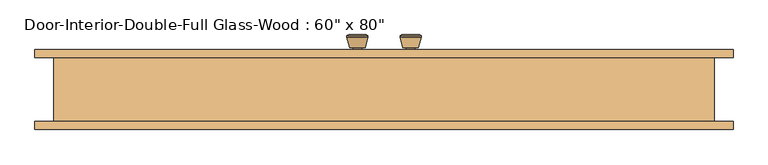
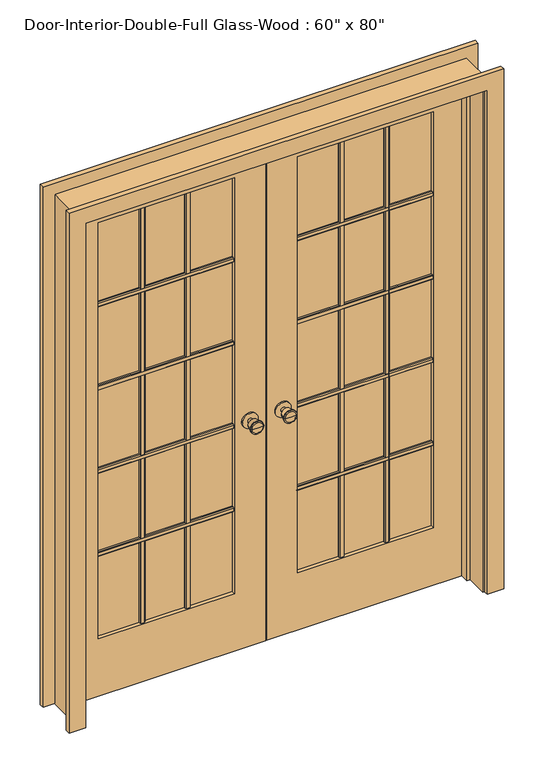
"""IFC4 building model written with IfcOpenShell, lengths in millimetres: door geometry."""

from ifc_helpers import new_model, si_unit, point, frame, frame_2d, origin, place, context, project, spatial, polyline, circle_curve, trimmed, segment, composite_curve, outline, extrude, faceted_brep, source, transform, mapped, element, save
from ifc_brep_helpers import plane_surface, cylinder_surface, revolved_surface, advanced_brep


def door_31a77bde(model_context):
    return source(origin(), model_context, "Body", "SolidModel", [
        advanced_brep(
        [(-63.5, 79.025, 914.4), (-73.5, 79.025, 914.4), (-53.5, 79.025, 914.4), (-83.9758676, 128.025, 914.4), (-63.5, 128.025, 914.4), (-43.0241324, 128.025, 914.4), (-88.5, 126.1971319, 914.4), (-38.5, 126.1971319, 914.4), (-88.5, 122.7334537, 914.4), (-38.5, 122.7334537, 914.4), (-82.136236, 98.025, 914.4), (-44.863764, 98.025, 914.4), (-73.5, 98.025, 914.4), (-53.5, 98.025, 914.4)],
        [
            (0, 1),
            (1, 2, circle_curve(frame((-63.5, 79.025, 914.4), z_axis=(0.0, -1.0, 0.0), x_axis=(1.0, 0.0, 0.0)), 10.0)),
            (2, 0),
            (2, 1, circle_curve(frame((-63.5, 79.025, 914.4), z_axis=(0.0, -1.0, 0.0), x_axis=(1.0, 0.0, 0.0)), 10.0)),
            (3, 4),
            (4, 5),
            (5, 3, circle_curve(frame((-63.5, 128.025, 914.4), z_axis=(0.0, 1.0, 0.0), x_axis=(1.0, 0.0, 0.0)), 20.4758676)),
            (3, 5, circle_curve(frame((-63.5, 128.025, 914.4), z_axis=(0.0, 1.0, 0.0), x_axis=(1.0, 0.0, 0.0)), 20.4758676)),
            (6, 3),
            (5, 7),
            (7, 6, circle_curve(frame((-63.5, 126.1971319, 914.4), z_axis=(0.0, 1.0, 0.0), x_axis=(1.0, 0.0, 0.0)), 25.0)),
            (6, 7, circle_curve(frame((-63.5, 126.1971319, 914.4), z_axis=(0.0, 1.0, 0.0), x_axis=(1.0, 0.0, 0.0)), 25.0)),
            (8, 6),
            (7, 9),
            (9, 8, circle_curve(frame((-63.5, 122.7334537, 914.4), z_axis=(0.0, 1.0, 0.0), x_axis=(1.0, 0.0, 0.0)), 25.0)),
            (8, 9, circle_curve(frame((-63.5, 122.7334537, 914.4), z_axis=(0.0, 1.0, 0.0), x_axis=(1.0, 0.0, 0.0)), 25.0)),
            (10, 8),
            (9, 11),
            (11, 10, circle_curve(frame((-63.5, 98.025, 914.4), z_axis=(0.0, 1.0, 0.0), x_axis=(1.0, 0.0, 0.0)), 18.636236)),
            (10, 11, circle_curve(frame((-63.5, 98.025, 914.4), z_axis=(0.0, 1.0, 0.0), x_axis=(1.0, 0.0, 0.0)), 18.636236)),
            (12, 10),
            (11, 13),
            (13, 12, circle_curve(frame((-63.5, 98.025, 914.4), z_axis=(0.0, 1.0, 0.0), x_axis=(1.0, 0.0, 0.0)), 10.0)),
            (12, 13, circle_curve(frame((-63.5, 98.025, 914.4), z_axis=(0.0, 1.0, 0.0), x_axis=(1.0, 0.0, 0.0)), 10.0)),
            (1, 12),
            (13, 2),
        ],
        [
            plane_surface(frame((-63.5, 79.025, 914.4), z_axis=(0.0, -1.0, 0.0), x_axis=(1.0, 0.0, 0.0))),
            plane_surface(frame((-63.5, 128.025, 914.4), z_axis=(0.0, 1.0, 0.0), x_axis=(1.0, 0.0, 0.0))),
            revolved_surface(polyline([(-43.0241324, 128.025, 914.4), (-38.5, 126.1971319, 914.4)]), (-63.5, 79.025, 914.4), (0.0, -1.0, 0.0)),
            cylinder_surface(frame((-63.5, 79.025, 914.4), z_axis=(0.0, -1.0, 0.0), x_axis=(1.0, 0.0, 0.0)), 25.0),
            revolved_surface(polyline([(-38.5, 122.7334537, 914.4), (-44.863764, 98.025, 914.4)]), (-63.5, 79.025, 914.4), (0.0, -1.0, 0.0)),
            plane_surface(frame((-63.5, 98.025, 914.4), z_axis=(0.0, -1.0, 0.0), x_axis=(1.0, 0.0, 0.0))),
            cylinder_surface(frame((-63.5, 79.025, 914.4), z_axis=(0.0, -1.0, 0.0), x_axis=(1.0, 0.0, 0.0)), 10.0),
        ],
        [
            (0, [[1, 2, 3]]),
            (0, [[-3, 4, -1]]),
            (1, [[5, 6, 7]]),
            (1, [[-6, -5, 8]]),
            (2, [[9, -7, 10, 11]]),
            (2, [[-10, -8, -9, 12]]),
            (3, [[13, -11, 14, 15]]),
            (3, [[-14, -12, -13, 16]]),
            (4, [[17, -15, 18, 19]]),
            (4, [[-18, -16, -17, 20]]),
            (5, [[21, -19, 22, 23]]),
            (5, [[-22, -20, -21, 24]]),
            (6, [[25, -23, 26, -2]]),
            (6, [[-26, -24, -25, -4]]),
        ],
    ),
        extrude(outline(composite_curve([segment(trimmed(circle_curve(frame_2d((914.4, -63.5)), 30.0), [point((914.4, -33.5))], [point((914.4, -93.5))], False, "CARTESIAN"), True, "CONTINUOUS"), segment(trimmed(circle_curve(frame_2d((914.4, -63.5)), 30.0), [point((914.4, -93.5))], [point((914.4, -33.5))], False, "CARTESIAN"), True, "CONTINUOUS")], self_intersect=False)), frame((0.0, 73.025, 0.0), z_axis=(0.0, 1.0, 0.0), x_axis=(0.0, 0.0, 1.0)), (0.0, 0.0, 1.0), 6.0),
        advanced_brep(
        [(-63.5, 32.1, 914.4), (-53.5, 32.1, 914.4), (-73.5, 32.1, 914.4), (-83.9758676, -16.9, 914.4), (-43.0241324, -16.9, 914.4), (-63.5, -16.9, 914.4), (-88.5, -15.0721319, 914.4), (-38.5, -15.0721319, 914.4), (-88.5, -11.6084537, 914.4), (-38.5, -11.6084537, 914.4), (-82.136236, 13.1, 914.4), (-44.863764, 13.1, 914.4), (-73.5, 13.1, 914.4), (-53.5, 13.1, 914.4)],
        [
            (0, 1),
            (1, 2, circle_curve(frame((-63.5, 32.1, 914.4), z_axis=(0.0, 1.0, 0.0), x_axis=(1.0, 0.0, 0.0)), 10.0)),
            (2, 0),
            (2, 1, circle_curve(frame((-63.5, 32.1, 914.4), z_axis=(0.0, 1.0, 0.0), x_axis=(1.0, 0.0, 0.0)), 10.0)),
            (3, 4, circle_curve(frame((-63.5, -16.9, 914.4), z_axis=(0.0, -1.0, 0.0), x_axis=(1.0, 0.0, 0.0)), 20.4758676)),
            (4, 5),
            (5, 3),
            (4, 3, circle_curve(frame((-63.5, -16.9, 914.4), z_axis=(0.0, -1.0, 0.0), x_axis=(1.0, 0.0, 0.0)), 20.4758676)),
            (6, 7, circle_curve(frame((-63.5, -15.0721319, 914.4), z_axis=(0.0, -1.0, 0.0), x_axis=(1.0, 0.0, 0.0)), 25.0)),
            (7, 4),
            (3, 6),
            (7, 6, circle_curve(frame((-63.5, -15.0721319, 914.4), z_axis=(0.0, -1.0, 0.0), x_axis=(1.0, 0.0, 0.0)), 25.0)),
            (8, 9, circle_curve(frame((-63.5, -11.6084537, 914.4), z_axis=(0.0, -1.0, 0.0), x_axis=(1.0, 0.0, 0.0)), 25.0)),
            (9, 7),
            (6, 8),
            (9, 8, circle_curve(frame((-63.5, -11.6084537, 914.4), z_axis=(0.0, -1.0, 0.0), x_axis=(1.0, 0.0, 0.0)), 25.0)),
            (10, 11, circle_curve(frame((-63.5, 13.1, 914.4), z_axis=(0.0, -1.0, 0.0), x_axis=(1.0, 0.0, 0.0)), 18.636236)),
            (11, 9),
            (8, 10),
            (11, 10, circle_curve(frame((-63.5, 13.1, 914.4), z_axis=(0.0, -1.0, 0.0), x_axis=(1.0, 0.0, 0.0)), 18.636236)),
            (12, 13, circle_curve(frame((-63.5, 13.1, 914.4), z_axis=(0.0, -1.0, 0.0), x_axis=(1.0, 0.0, 0.0)), 10.0)),
            (13, 11),
            (10, 12),
            (13, 12, circle_curve(frame((-63.5, 13.1, 914.4), z_axis=(0.0, -1.0, 0.0), x_axis=(1.0, 0.0, 0.0)), 10.0)),
            (1, 13),
            (12, 2),
        ],
        [
            plane_surface(frame((-63.5, 32.1, 914.4), z_axis=(0.0, 1.0, 0.0), x_axis=(1.0, 0.0, 0.0))),
            plane_surface(frame((-63.5, -16.9, 914.4), z_axis=(0.0, -1.0, 0.0), x_axis=(1.0, 0.0, 0.0))),
            revolved_surface(polyline([(-43.0241324, -16.9, 914.4), (-38.5, -15.0721319, 914.4)]), (-63.5, 32.1, 914.4), (0.0, 1.0, 0.0)),
            cylinder_surface(frame((-63.5, 32.1, 914.4), z_axis=(0.0, 1.0, 0.0), x_axis=(1.0, 0.0, 0.0)), 25.0),
            revolved_surface(polyline([(-38.5, -11.6084537, 914.4), (-44.863764, 13.1, 914.4)]), (-63.5, 32.1, 914.4), (0.0, 1.0, 0.0)),
            plane_surface(frame((-63.5, 13.1, 914.4), z_axis=(0.0, 1.0, 0.0), x_axis=(1.0, 0.0, 0.0))),
            cylinder_surface(frame((-63.5, 32.1, 914.4), z_axis=(0.0, 1.0, 0.0), x_axis=(1.0, 0.0, 0.0)), 10.0),
        ],
        [
            (0, [[1, 2, 3]]),
            (0, [[-3, 4, -1]]),
            (1, [[5, 6, 7]]),
            (1, [[8, -7, -6]]),
            (2, [[9, 10, -5, 11]]),
            (2, [[12, -11, -8, -10]]),
            (3, [[13, 14, -9, 15]]),
            (3, [[16, -15, -12, -14]]),
            (4, [[17, 18, -13, 19]]),
            (4, [[20, -19, -16, -18]]),
            (5, [[21, 22, -17, 23]]),
            (5, [[24, -23, -20, -22]]),
            (6, [[-2, 25, -21, 26]]),
            (6, [[-4, -26, -24, -25]]),
        ],
    ),
        extrude(outline(composite_curve([segment(trimmed(circle_curve(frame_2d((914.4, -63.5)), 30.0), [point((914.4, -33.5))], [point((914.4, -93.5))], False, "CARTESIAN"), True, "CONTINUOUS"), segment(trimmed(circle_curve(frame_2d((914.4, -63.5)), 30.0), [point((914.4, -93.5))], [point((914.4, -33.5))], False, "CARTESIAN"), True, "CONTINUOUS")], self_intersect=False)), frame((0.0, 32.1, 0.0), z_axis=(0.0, 1.0, 0.0), x_axis=(0.0, 0.0, 1.0)), (0.0, 0.0, 1.0), 6.0),
        extrude(outline(polyline([(52.07, 1586.23), (52.07, 1567.18), (45.72, 1567.18), (42.545, 1570.355), (42.545, 1583.055), (45.72, 1586.23), (52.07, 1586.23)])), frame((120.65, 0.0, 0.0), z_axis=(1.0, 0.0, 0.0), x_axis=(0.0, 1.0, 0.0)), (0.0, 0.0, 1.0), 520.7),
        extrude(outline(polyline([(52.07, 1249.9975), (52.07, 1230.9475), (45.72, 1230.9475), (42.545, 1234.1225), (42.545, 1246.8225), (45.72, 1249.9975), (52.07, 1249.9975)])), frame((120.65, 0.0, 0.0), z_axis=(1.0, 0.0, 0.0), x_axis=(0.0, 1.0, 0.0)), (0.0, 0.0, 1.0), 520.7),
        extrude(outline(polyline([(52.07, 913.765), (52.07, 894.715), (45.72, 894.715), (42.545, 897.89), (42.545, 910.59), (45.72, 913.765), (52.07, 913.765)])), frame((120.65, 0.0, 0.0), z_axis=(1.0, 0.0, 0.0), x_axis=(0.0, 1.0, 0.0)), (0.0, 0.0, 1.0), 520.7),
        extrude(outline(polyline([(52.07, 577.5325), (52.07, 558.4825), (45.72, 558.4825), (42.545, 561.6575), (42.545, 574.3575), (45.72, 577.5325), (52.07, 577.5325)])), frame((120.65, 0.0, 0.0), z_axis=(1.0, 0.0, 0.0), x_axis=(0.0, 1.0, 0.0)), (0.0, 0.0, 1.0), 520.7),
        extrude(outline(polyline([(458.2583333, 52.07), (477.3083333, 52.07), (477.3083333, 45.72), (474.1333333, 42.545), (461.4333333, 42.545), (458.2583333, 45.72), (458.2583333, 52.07)])), frame((0.0, 0.0, 231.775), z_axis=(0.0, 0.0, 1.0), x_axis=(1.0, 0.0, 0.0)), (0.0, 0.0, 1.0), 1681.1625),
        extrude(outline(polyline([(284.6916667, 52.07), (303.7416667, 52.07), (303.7416667, 45.72), (300.5666667, 42.545), (287.8666667, 42.545), (284.6916667, 45.72), (284.6916667, 52.07)])), frame((0.0, 0.0, 231.775), z_axis=(0.0, 0.0, 1.0), x_axis=(1.0, 0.0, 0.0)), (0.0, 0.0, 1.0), 1681.1625),
        extrude(outline(polyline([(59.055, 1586.23), (65.405, 1586.23), (68.58, 1583.055), (68.58, 1570.355), (65.405, 1567.18), (59.055, 1567.18), (59.055, 1586.23)])), frame((-641.35, 0.0, 0.0), z_axis=(1.0, 0.0, 0.0), x_axis=(0.0, 1.0, 0.0)), (0.0, 0.0, 1.0), 520.7),
        extrude(outline(polyline([(59.055, 1249.9975), (65.405, 1249.9975), (68.58, 1246.8225), (68.58, 1234.1225), (65.405, 1230.9475), (59.055, 1230.9475), (59.055, 1249.9975)])), frame((-641.35, 0.0, 0.0), z_axis=(1.0, 0.0, 0.0), x_axis=(0.0, 1.0, 0.0)), (0.0, 0.0, 1.0), 520.7),
        extrude(outline(polyline([(59.055, 913.765), (65.405, 913.765), (68.58, 910.59), (68.58, 897.89), (65.405, 894.715), (59.055, 894.715), (59.055, 913.765)])), frame((-641.35, 0.0, 0.0), z_axis=(1.0, 0.0, 0.0), x_axis=(0.0, 1.0, 0.0)), (0.0, 0.0, 1.0), 520.7),
        extrude(outline(polyline([(59.055, 577.5325), (65.405, 577.5325), (68.58, 574.3575), (68.58, 561.6575), (65.405, 558.4825), (59.055, 558.4825), (59.055, 577.5325)])), frame((-641.35, 0.0, 0.0), z_axis=(1.0, 0.0, 0.0), x_axis=(0.0, 1.0, 0.0)), (0.0, 0.0, 1.0), 520.7),
        extrude(outline(polyline([(-303.7416667, 59.055), (-303.7416667, 65.405), (-300.5666667, 68.58), (-287.8666667, 68.58), (-284.6916667, 65.405), (-284.6916667, 59.055), (-303.7416667, 59.055)])), frame((0.0, 0.0, 231.775), z_axis=(0.0, 0.0, 1.0), x_axis=(1.0, 0.0, 0.0)), (0.0, 0.0, 1.0), 1681.1625),
        extrude(outline(polyline([(-477.3083333, 59.055), (-477.3083333, 65.405), (-474.1333333, 68.58), (-461.4333333, 68.58), (-458.2583333, 65.405), (-458.2583333, 59.055), (-477.3083333, 59.055)])), frame((0.0, 0.0, 231.775), z_axis=(0.0, 0.0, 1.0), x_axis=(1.0, 0.0, 0.0)), (0.0, 0.0, 1.0), 1681.1625),
        extrude(outline(polyline([(59.055, 1586.23), (65.405, 1586.23), (68.58, 1583.055), (68.58, 1570.355), (65.405, 1567.18), (59.055, 1567.18), (59.055, 1586.23)])), frame((120.65, 0.0, 0.0), z_axis=(1.0, 0.0, 0.0), x_axis=(0.0, 1.0, 0.0)), (0.0, 0.0, 1.0), 520.7),
        extrude(outline(polyline([(59.055, 1249.9975), (65.405, 1249.9975), (68.58, 1246.8225), (68.58, 1234.1225), (65.405, 1230.9475), (59.055, 1230.9475), (59.055, 1249.9975)])), frame((120.65, 0.0, 0.0), z_axis=(1.0, 0.0, 0.0), x_axis=(0.0, 1.0, 0.0)), (0.0, 0.0, 1.0), 520.7),
        extrude(outline(polyline([(59.055, 913.765), (65.405, 913.765), (68.58, 910.59), (68.58, 897.89), (65.405, 894.715), (59.055, 894.715), (59.055, 913.765)])), frame((120.65, 0.0, 0.0), z_axis=(1.0, 0.0, 0.0), x_axis=(0.0, 1.0, 0.0)), (0.0, 0.0, 1.0), 520.7),
        extrude(outline(polyline([(59.055, 577.5325), (65.405, 577.5325), (68.58, 574.3575), (68.58, 561.6575), (65.405, 558.4825), (59.055, 558.4825), (59.055, 577.5325)])), frame((120.65, 0.0, 0.0), z_axis=(1.0, 0.0, 0.0), x_axis=(0.0, 1.0, 0.0)), (0.0, 0.0, 1.0), 520.7),
        extrude(outline(polyline([(458.2583333, 59.055), (458.2583333, 65.405), (461.4333333, 68.58), (474.1333333, 68.58), (477.3083333, 65.405), (477.3083333, 59.055), (458.2583333, 59.055)])), frame((0.0, 0.0, 231.775), z_axis=(0.0, 0.0, 1.0), x_axis=(1.0, 0.0, 0.0)), (0.0, 0.0, 1.0), 1681.1625),
        extrude(outline(polyline([(284.6916667, 59.055), (284.6916667, 65.405), (287.8666667, 68.58), (300.5666667, 68.58), (303.7416667, 65.405), (303.7416667, 59.055), (284.6916667, 59.055)])), frame((0.0, 0.0, 231.775), z_axis=(0.0, 0.0, 1.0), x_axis=(1.0, 0.0, 0.0)), (0.0, 0.0, 1.0), 1681.1625),
        extrude(outline(polyline([(52.07, 1586.23), (52.07, 1567.18), (45.72, 1567.18), (42.545, 1570.355), (42.545, 1583.055), (45.72, 1586.23), (52.07, 1586.23)])), frame((-641.35, 0.0, 0.0), z_axis=(1.0, 0.0, 0.0), x_axis=(0.0, 1.0, 0.0)), (0.0, 0.0, 1.0), 520.7),
        extrude(outline(polyline([(52.07, 1249.9975), (52.07, 1230.9475), (45.72, 1230.9475), (42.545, 1234.1225), (42.545, 1246.8225), (45.72, 1249.9975), (52.07, 1249.9975)])), frame((-641.35, 0.0, 0.0), z_axis=(1.0, 0.0, 0.0), x_axis=(0.0, 1.0, 0.0)), (0.0, 0.0, 1.0), 520.7),
        extrude(outline(polyline([(52.07, 913.765), (52.07, 894.715), (45.72, 894.715), (42.545, 897.89), (42.545, 910.59), (45.72, 913.765), (52.07, 913.765)])), frame((-641.35, 0.0, 0.0), z_axis=(1.0, 0.0, 0.0), x_axis=(0.0, 1.0, 0.0)), (0.0, 0.0, 1.0), 520.7),
        extrude(outline(polyline([(52.07, 577.5325), (52.07, 558.4825), (45.72, 558.4825), (42.545, 561.6575), (42.545, 574.3575), (45.72, 577.5325), (52.07, 577.5325)])), frame((-641.35, 0.0, 0.0), z_axis=(1.0, 0.0, 0.0), x_axis=(0.0, 1.0, 0.0)), (0.0, 0.0, 1.0), 520.7),
        extrude(outline(polyline([(-303.7416667, 52.07), (-284.6916667, 52.07), (-284.6916667, 45.72), (-287.8666667, 42.545), (-300.5666667, 42.545), (-303.7416667, 45.72), (-303.7416667, 52.07)])), frame((0.0, 0.0, 231.775), z_axis=(0.0, 0.0, 1.0), x_axis=(1.0, 0.0, 0.0)), (0.0, 0.0, 1.0), 1681.1625),
        extrude(outline(polyline([(-477.3083333, 52.07), (-458.2583333, 52.07), (-458.2583333, 45.72), (-461.4333333, 42.545), (-474.1333333, 42.545), (-477.3083333, 45.72), (-477.3083333, 52.07)])), frame((0.0, 0.0, 231.775), z_axis=(0.0, 0.0, 1.0), x_axis=(1.0, 0.0, 0.0)), (0.0, 0.0, 1.0), 1681.1625),
        advanced_brep(
        [(63.5, 32.1, 914.4), (73.5, 32.1, 914.4), (53.5, 32.1, 914.4), (83.9758676, -16.9, 914.4), (63.5, -16.9, 914.4), (43.0241324, -16.9, 914.4), (88.5, -15.0721319, 914.4), (38.5, -15.0721319, 914.4), (88.5, -11.6084537, 914.4), (38.5, -11.6084537, 914.4), (82.136236, 13.1, 914.4), (44.863764, 13.1, 914.4), (73.5, 13.1, 914.4), (53.5, 13.1, 914.4)],
        [
            (0, 1),
            (1, 2, circle_curve(frame((63.5, 32.1, 914.4), z_axis=(0.0, 1.0, 0.0), x_axis=(-1.0, 0.0, 0.0)), 10.0)),
            (2, 0),
            (2, 1, circle_curve(frame((63.5, 32.1, 914.4), z_axis=(0.0, 1.0, 0.0), x_axis=(-1.0, 0.0, 0.0)), 10.0)),
            (3, 4),
            (4, 5),
            (5, 3, circle_curve(frame((63.5, -16.9, 914.4), z_axis=(0.0, -1.0, 0.0), x_axis=(-1.0, 0.0, 0.0)), 20.4758676)),
            (3, 5, circle_curve(frame((63.5, -16.9, 914.4), z_axis=(0.0, -1.0, 0.0), x_axis=(-1.0, 0.0, 0.0)), 20.4758676)),
            (6, 3),
            (5, 7),
            (7, 6, circle_curve(frame((63.5, -15.0721319, 914.4), z_axis=(0.0, -1.0, 0.0), x_axis=(-1.0, 0.0, 0.0)), 25.0)),
            (6, 7, circle_curve(frame((63.5, -15.0721319, 914.4), z_axis=(0.0, -1.0, 0.0), x_axis=(-1.0, 0.0, 0.0)), 25.0)),
            (8, 6),
            (7, 9),
            (9, 8, circle_curve(frame((63.5, -11.6084537, 914.4), z_axis=(0.0, -1.0, 0.0), x_axis=(-1.0, 0.0, 0.0)), 25.0)),
            (8, 9, circle_curve(frame((63.5, -11.6084537, 914.4), z_axis=(0.0, -1.0, 0.0), x_axis=(-1.0, 0.0, 0.0)), 25.0)),
            (10, 8),
            (9, 11),
            (11, 10, circle_curve(frame((63.5, 13.1, 914.4), z_axis=(0.0, -1.0, 0.0), x_axis=(-1.0, 0.0, 0.0)), 18.636236)),
            (10, 11, circle_curve(frame((63.5, 13.1, 914.4), z_axis=(0.0, -1.0, 0.0), x_axis=(-1.0, 0.0, 0.0)), 18.636236)),
            (12, 10),
            (11, 13),
            (13, 12, circle_curve(frame((63.5, 13.1, 914.4), z_axis=(0.0, -1.0, 0.0), x_axis=(-1.0, 0.0, 0.0)), 10.0)),
            (12, 13, circle_curve(frame((63.5, 13.1, 914.4), z_axis=(0.0, -1.0, 0.0), x_axis=(-1.0, 0.0, 0.0)), 10.0)),
            (1, 12),
            (13, 2),
        ],
        [
            plane_surface(frame((63.5, 32.1, 914.4), z_axis=(0.0, 1.0, 0.0), x_axis=(-1.0, 0.0, 0.0))),
            plane_surface(frame((63.5, -16.9, 914.4), z_axis=(0.0, -1.0, 0.0), x_axis=(-1.0, 0.0, 0.0))),
            revolved_surface(polyline([(43.0241324, -16.9, 914.4), (38.5, -15.0721319, 914.4)]), (63.5, 32.1, 914.4), (0.0, 1.0, 0.0)),
            cylinder_surface(frame((63.5, 32.1, 914.4), z_axis=(0.0, 1.0, 0.0), x_axis=(-1.0, 0.0, 0.0)), 25.0),
            revolved_surface(polyline([(38.5, -11.6084537, 914.4), (44.863764, 13.1, 914.4)]), (63.5, 32.1, 914.4), (0.0, 1.0, 0.0)),
            plane_surface(frame((63.5, 13.1, 914.4), z_axis=(0.0, 1.0, 0.0), x_axis=(-1.0, 0.0, 0.0))),
            cylinder_surface(frame((63.5, 32.1, 914.4), z_axis=(0.0, 1.0, 0.0), x_axis=(-1.0, 0.0, 0.0)), 10.0),
        ],
        [
            (0, [[1, 2, 3]]),
            (0, [[-3, 4, -1]]),
            (1, [[5, 6, 7]]),
            (1, [[-6, -5, 8]]),
            (2, [[9, -7, 10, 11]]),
            (2, [[-10, -8, -9, 12]]),
            (3, [[13, -11, 14, 15]]),
            (3, [[-14, -12, -13, 16]]),
            (4, [[17, -15, 18, 19]]),
            (4, [[-18, -16, -17, 20]]),
            (5, [[21, -19, 22, 23]]),
            (5, [[-22, -20, -21, 24]]),
            (6, [[25, -23, 26, -2]]),
            (6, [[-26, -24, -25, -4]]),
        ],
    ),
        extrude(outline(composite_curve([segment(trimmed(circle_curve(frame_2d((914.4, 63.5)), 30.0), [point((914.4, 33.5))], [point((914.4, 93.5))], False, "CARTESIAN"), True, "CONTINUOUS"), segment(trimmed(circle_curve(frame_2d((914.4, 63.5)), 30.0), [point((914.4, 93.5))], [point((914.4, 33.5))], False, "CARTESIAN"), True, "CONTINUOUS")], self_intersect=False)), frame((0.0, 32.1, 0.0), z_axis=(0.0, 1.0, 0.0), x_axis=(0.0, 0.0, 1.0)), (0.0, 0.0, 1.0), 6.0),
        advanced_brep(
        [(63.5, 79.025, 914.4), (53.5, 79.025, 914.4), (73.5, 79.025, 914.4), (83.9758676, 128.025, 914.4), (43.0241324, 128.025, 914.4), (63.5, 128.025, 914.4), (88.5, 126.1971319, 914.4), (38.5, 126.1971319, 914.4), (88.5, 122.7334537, 914.4), (38.5, 122.7334537, 914.4), (82.136236, 98.025, 914.4), (44.863764, 98.025, 914.4), (73.5, 98.025, 914.4), (53.5, 98.025, 914.4)],
        [
            (0, 1),
            (1, 2, circle_curve(frame((63.5, 79.025, 914.4), z_axis=(0.0, -1.0, 0.0), x_axis=(-1.0, 0.0, 0.0)), 10.0)),
            (2, 0),
            (2, 1, circle_curve(frame((63.5, 79.025, 914.4), z_axis=(0.0, -1.0, 0.0), x_axis=(-1.0, 0.0, 0.0)), 10.0)),
            (3, 4, circle_curve(frame((63.5, 128.025, 914.4), z_axis=(0.0, 1.0, 0.0), x_axis=(-1.0, 0.0, 0.0)), 20.4758676)),
            (4, 5),
            (5, 3),
            (4, 3, circle_curve(frame((63.5, 128.025, 914.4), z_axis=(0.0, 1.0, 0.0), x_axis=(-1.0, 0.0, 0.0)), 20.4758676)),
            (6, 7, circle_curve(frame((63.5, 126.1971319, 914.4), z_axis=(0.0, 1.0, 0.0), x_axis=(-1.0, 0.0, 0.0)), 25.0)),
            (7, 4),
            (3, 6),
            (7, 6, circle_curve(frame((63.5, 126.1971319, 914.4), z_axis=(0.0, 1.0, 0.0), x_axis=(-1.0, 0.0, 0.0)), 25.0)),
            (8, 9, circle_curve(frame((63.5, 122.7334537, 914.4), z_axis=(0.0, 1.0, 0.0), x_axis=(-1.0, 0.0, 0.0)), 25.0)),
            (9, 7),
            (6, 8),
            (9, 8, circle_curve(frame((63.5, 122.7334537, 914.4), z_axis=(0.0, 1.0, 0.0), x_axis=(-1.0, 0.0, 0.0)), 25.0)),
            (10, 11, circle_curve(frame((63.5, 98.025, 914.4), z_axis=(0.0, 1.0, 0.0), x_axis=(-1.0, 0.0, 0.0)), 18.636236)),
            (11, 9),
            (8, 10),
            (11, 10, circle_curve(frame((63.5, 98.025, 914.4), z_axis=(0.0, 1.0, 0.0), x_axis=(-1.0, 0.0, 0.0)), 18.636236)),
            (12, 13, circle_curve(frame((63.5, 98.025, 914.4), z_axis=(0.0, 1.0, 0.0), x_axis=(-1.0, 0.0, 0.0)), 10.0)),
            (13, 11),
            (10, 12),
            (13, 12, circle_curve(frame((63.5, 98.025, 914.4), z_axis=(0.0, 1.0, 0.0), x_axis=(-1.0, 0.0, 0.0)), 10.0)),
            (1, 13),
            (12, 2),
        ],
        [
            plane_surface(frame((63.5, 79.025, 914.4), z_axis=(0.0, -1.0, 0.0), x_axis=(-1.0, 0.0, 0.0))),
            plane_surface(frame((63.5, 128.025, 914.4), z_axis=(0.0, 1.0, 0.0), x_axis=(-1.0, 0.0, 0.0))),
            revolved_surface(polyline([(43.0241324, 128.025, 914.4), (38.5, 126.1971319, 914.4)]), (63.5, 79.025, 914.4), (0.0, -1.0, 0.0)),
            cylinder_surface(frame((63.5, 79.025, 914.4), z_axis=(0.0, -1.0, 0.0), x_axis=(-1.0, 0.0, 0.0)), 25.0),
            revolved_surface(polyline([(38.5, 122.7334537, 914.4), (44.863764, 98.025, 914.4)]), (63.5, 79.025, 914.4), (0.0, -1.0, 0.0)),
            plane_surface(frame((63.5, 98.025, 914.4), z_axis=(0.0, -1.0, 0.0), x_axis=(-1.0, 0.0, 0.0))),
            cylinder_surface(frame((63.5, 79.025, 914.4), z_axis=(0.0, -1.0, 0.0), x_axis=(-1.0, 0.0, 0.0)), 10.0),
        ],
        [
            (0, [[1, 2, 3]]),
            (0, [[-3, 4, -1]]),
            (1, [[5, 6, 7]]),
            (1, [[8, -7, -6]]),
            (2, [[9, 10, -5, 11]]),
            (2, [[12, -11, -8, -10]]),
            (3, [[13, 14, -9, 15]]),
            (3, [[16, -15, -12, -14]]),
            (4, [[17, 18, -13, 19]]),
            (4, [[20, -19, -16, -18]]),
            (5, [[21, 22, -17, 23]]),
            (5, [[24, -23, -20, -22]]),
            (6, [[-2, 25, -21, 26]]),
            (6, [[-4, -26, -24, -25]]),
        ],
    ),
        extrude(outline(composite_curve([segment(trimmed(circle_curve(frame_2d((914.4, 63.5)), 30.0), [point((914.4, 33.5))], [point((914.4, 93.5))], False, "CARTESIAN"), True, "CONTINUOUS"), segment(trimmed(circle_curve(frame_2d((914.4, 63.5)), 30.0), [point((914.4, 93.5))], [point((914.4, 33.5))], False, "CARTESIAN"), True, "CONTINUOUS")], self_intersect=False)), frame((0.0, 73.025, 0.0), z_axis=(0.0, 1.0, 0.0), x_axis=(0.0, 0.0, 1.0)), (0.0, 0.0, 1.0), 6.0),
        extrude(outline(polyline([(0.0, 768.35), (0.0, 831.85), (2101.85, 831.85), (2101.85, -831.85), (0.0, -831.85), (0.0, -768.35), (2038.35, -768.35), (2038.35, 768.35), (0.0, 768.35)])), frame((0.0, 73.025, 0.0), z_axis=(0.0, 1.0, 0.0), x_axis=(0.0, 0.0, 1.0)), (0.0, 0.0, 1.0), 19.05),
        extrude(outline(polyline([(0.0, 768.35), (0.0, 831.85), (2101.85, 831.85), (2101.85, -831.85), (0.0, -831.85), (0.0, -768.35), (2038.35, -768.35), (2038.35, 768.35), (0.0, 768.35)])), frame((0.0, -98.425, 0.0), z_axis=(0.0, 1.0, 0.0), x_axis=(0.0, 0.0, 1.0)), (0.0, 0.0, 1.0), 19.05),
        extrude(outline(polyline([(2032.0, -762.0), (0.0, -762.0), (0.0, -1.6019111), (2032.0, -1.6019111), (2032.0, -762.0)]), holes=[polyline([(231.775, -641.35), (1912.9375, -641.35), (1912.9375, -120.65), (231.775, -120.65), (231.775, -641.35)])]), frame((0.0, 38.1, 0.0), z_axis=(0.0, 1.0, 0.0), x_axis=(0.0, 0.0, 1.0)), (0.0, 0.0, 1.0), 34.925),
        extrude(outline(polyline([(0.0, 762.0), (2032.0, 762.0), (2032.0, 1.5875), (0.0, 1.5875), (0.0, 762.0)]), holes=[polyline([(1912.9375, 120.65), (1912.9375, 641.35), (231.775, 641.35), (231.775, 120.65), (1912.9375, 120.65)])]), frame((0.0, 38.1, 0.0), z_axis=(0.0, 1.0, 0.0), x_axis=(0.0, 0.0, 1.0)), (0.0, 0.0, 1.0), 34.925),
        faceted_brep([(787.4, 73.025, 0.0), (787.4, -79.375, 0.0), (762.0, -79.375, 0.0), (762.0, 3.175, 0.0), (749.3, 3.175, 0.0), (749.3, 38.1, 0.0), (762.0, 38.1, 0.0), (762.0, 73.025, 0.0), (787.4, 73.025, 2057.4), (787.4, -79.375, 2057.4), (-787.4, -79.375, 2057.4), (-787.4, -79.375, 0.0), (-762.0, -79.375, 0.0), (-762.0, -79.375, 2032.0), (762.0, -79.375, 2032.0), (762.0, 3.175, 2032.0), (-762.0, 3.175, 2032.0), (-762.0, 3.175, 0.0), (-749.3, 3.175, 0.0), (-749.3, 3.175, 2019.3), (749.3, 3.175, 2019.3), (749.3, 38.1, 2019.3), (1.5875, 38.1, 2019.3), (-1.6019111, 38.1, 2019.3), (-749.3, 38.1, 2019.3), (-749.3, 38.1, 0.0), (-762.0, 38.1, 0.0), (-762.0, 38.1, 2032.0), (-1.6019111, 38.1, 2032.0), (1.5875, 38.1, 2032.0), (762.0, 38.1, 2032.0), (762.0, 73.025, 2032.0), (1.5875, 73.025, 2032.0), (-1.6019111, 73.025, 2032.0), (-762.0, 73.025, 2032.0), (-762.0, 73.025, 0.0), (-787.4, 73.025, 0.0), (-787.4, 73.025, 2057.4)], [[[0, 1, 2, 3, 4, 5, 6, 7]], [[1, 0, 8, 9]], [[2, 1, 9, 10, 11, 12, 13, 14]], [[3, 2, 14, 15]], [[4, 3, 15, 16, 17, 18, 19, 20]], [[5, 4, 20, 21]], [[6, 5, 21, 22, 23, 24, 25, 26, 27, 28, 29, 30]], [[7, 6, 30, 31]], [[0, 7, 31, 32, 33, 34, 35, 36, 37, 8]], [[9, 8, 37, 10]], [[14, 13, 16, 15]], [[20, 19, 24, 23, 22, 21]], [[31, 30, 29, 28, 27, 34, 33, 32]], [[12, 11, 36, 35, 26, 25, 18, 17]], [[11, 10, 37, 36]], [[13, 12, 17, 16]], [[19, 18, 25, 24]], [[27, 26, 35, 34]]]),
        extrude(outline(polyline([(641.35, 52.07), (120.65, 52.07), (120.65, 59.055), (641.35, 59.055), (641.35, 52.07)])), frame((0.0, 0.0, 231.775), z_axis=(0.0, 0.0, 1.0), x_axis=(1.0, 0.0, 0.0)), (0.0, 0.0, 1.0), 1681.1625),
        extrude(outline(polyline([(-120.65, 52.07), (-641.35, 52.07), (-641.35, 59.055), (-120.65, 59.055), (-120.65, 52.07)])), frame((0.0, 0.0, 231.775), z_axis=(0.0, 0.0, 1.0), x_axis=(1.0, 0.0, 0.0)), (0.0, 0.0, 1.0), 1681.1625),
    ])


if __name__ == "__main__":
    model = new_model("IFC4")
    model_context = context("Model", 3, world=origin())
    ifc_project = project(units=[si_unit("LENGTHUNIT", "METRE", prefix="MILLI")], contexts=[model_context])
    site = spatial("IfcSite", under=ifc_project)
    building = spatial("IfcBuilding", under=site)
    placement = place(None, origin())
    door_shape = door_31a77bde(model_context)
    element("IfcDoor", 1, ObjectType="Door-Interior-Double-Full Glass-Wood : 60\" x 80\"", at=placement, inside=building, context=model_context, shape_type="MappedRepresentation", body=[
        mapped(door_shape, transform((0.0, 0.0, 0.0), x_axis=(1.0, 0.0, 0.0), y_axis=(0.0, 1.0, 0.0), z_axis=(0.0, 0.0, 1.0))),
    ])
    save(model, "model.ifc")

# Revit data of these elements
# Type "Door-Interior-Double-Full Glass-Wood : 60\" x 80\""
#   Type Mark = "10"
#   Assembly Code = "C1020300"
#   Analytic Construction = "French door, wood frame with single glass"
#   Top Rail = 0' - 4 11/16"
#   Thickness = 0' - 1 3/8"
#   Thermal Resistance (R) = 1.0696 (h·ft²·°F)/BTU
#   Swing Angle [instance default] = 90.00°
#   Stiles = 0' - 4 3/4"
#   Rough Width = 5' - 2"
#   Rough Height = 6' - 9"
#   Panel Width = 2' - 6"
#   Height = 6' - 8"
#   Width = 5' - 0"
#   Heat Transfer Coefficient (U) = 0.9350 BTU/(h·ft²·°F)
#   Bottom Rail = 0' - 9 1/8"
#   Show Grill [instance default] = yes
#   Trim Material = Cherry
#   Panel Material = Cherry
#   Frame Material = Cherry
#   Door Handle Material = Aluminum
#   Visual Light Transmittance = 0
#   Solar Heat Gain Coefficient = 0
#   Wall Closure = (empty or 0)
#   Function = (empty or 0)
# Element 1 (IfcDoor, "Door-Interior-Double-Full Glass-Wood : 60\" x 80\"")
#   Materials on its faces: "Cherry", "Aluminum", "Glass"
# Materials
#   "Cherry": class "Wood", colour RGB 226 177 128, transparency 0, Description = "Prunus Serotina", Cost = 0
#   "Aluminum": class "Metal", colour RGB 247 247 247, transparency 0, Description = "Aluminum 6061", Cost = 0
#   "Glass": class "Glass", colour RGB 0 128 192, transparency 0.75, Description = "Soda Lime Glass", Cost = 0
